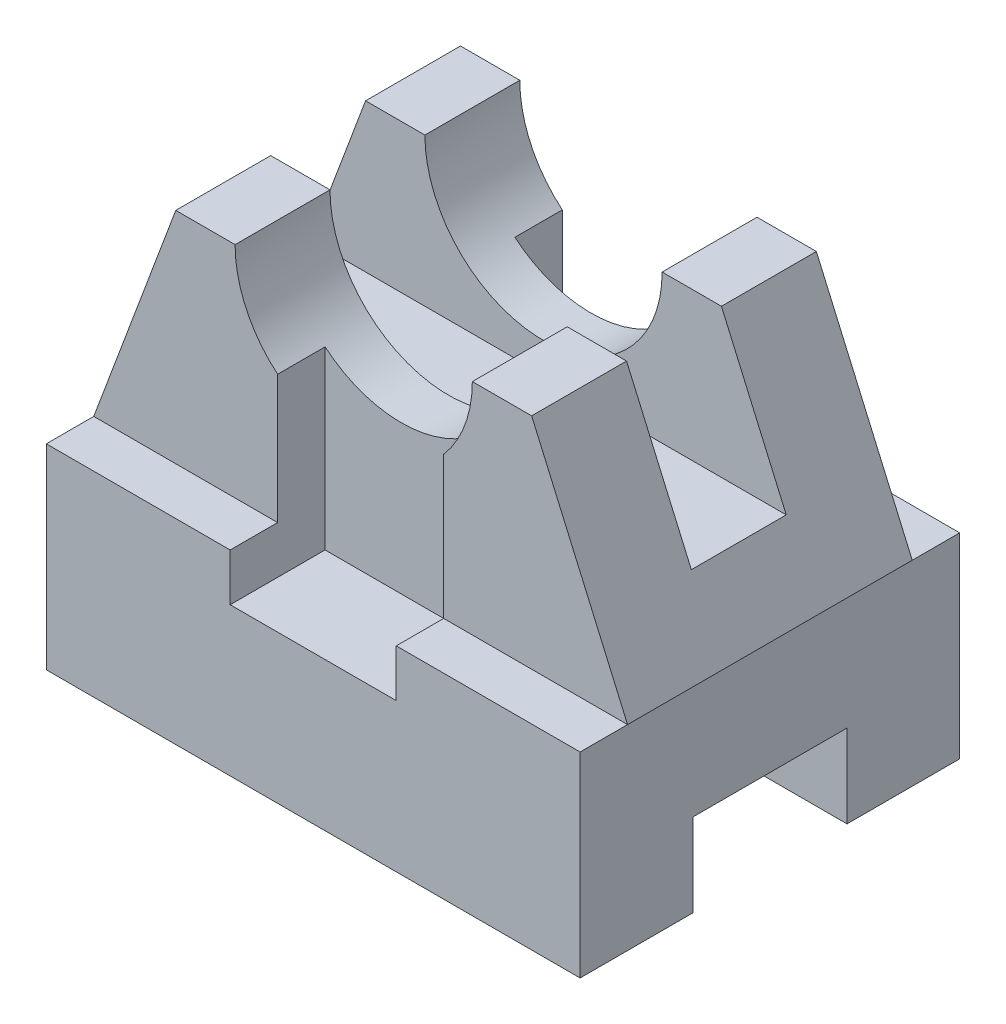
ISO-10303-21;
HEADER;
FILE_DESCRIPTION(('STEP AP214'),'2;1');
FILE_NAME('part.step','',(''),(''),'','','');
FILE_SCHEMA(('AUTOMOTIVE_DESIGN { 1 0 10303 214 1 1 1 1 }'));
ENDSEC;
DATA;
#1=APPLICATION_CONTEXT('core data for automotive mechanical design processes');
#2=APPLICATION_PROTOCOL_DEFINITION('international standard','automotive_design',2000,#1);
#3=PRODUCT_CONTEXT('',#1,'mechanical');
#4=PRODUCT('Part','Part','',(#3));
#5=PRODUCT_RELATED_PRODUCT_CATEGORY('part','',(#4));
#6=PRODUCT_DEFINITION_FORMATION('','',#4);
#7=PRODUCT_DEFINITION_CONTEXT('part definition',#1,'design');
#8=PRODUCT_DEFINITION('design','',#6,#7);
#9=PRODUCT_DEFINITION_SHAPE('','',#8);
#10=(LENGTH_UNIT() NAMED_UNIT(*) SI_UNIT(.MILLI.,.METRE.));
#11=(NAMED_UNIT(*) PLANE_ANGLE_UNIT() SI_UNIT($,.RADIAN.));
#12=(NAMED_UNIT(*) SI_UNIT($,.STERADIAN.) SOLID_ANGLE_UNIT());
#13=UNCERTAINTY_MEASURE_WITH_UNIT(LENGTH_MEASURE(1.E-05),#10,'distance_accuracy_value','');
#14=(GEOMETRIC_REPRESENTATION_CONTEXT(3) GLOBAL_UNCERTAINTY_ASSIGNED_CONTEXT((#13)) GLOBAL_UNIT_ASSIGNED_CONTEXT((#10,
#11,#12)) REPRESENTATION_CONTEXT('',''));
#15=CARTESIAN_POINT('',(0.,0.,0.));
#16=DIRECTION('',(0.,0.,1.));
#17=DIRECTION('',(1.,0.,0.));
#18=AXIS2_PLACEMENT_3D('',#15,#16,#17);
#19=CARTESIAN_POINT('',(0.,33.,32.));
#20=DIRECTION('',(0.,-1.,0.));
#21=DIRECTION('',(0.,0.,-1.));
#22=AXIS2_PLACEMENT_3D('',#19,#20,#21);
#23=PLANE('',#22);
#24=DIRECTION('',(-1.,0.,0.));
#25=VECTOR('',#24,1.);
#26=CARTESIAN_POINT('',(0.,33.,32.));
#27=LINE('',#26,#25);
#28=CARTESIAN_POINT('',(31.,33.,32.));
#29=VERTEX_POINT('',#28);
#30=CARTESIAN_POINT('',(0.,33.,32.));
#31=VERTEX_POINT('',#30);
#32=EDGE_CURVE('E433',#29,#31,#27,.T.);
#33=ORIENTED_EDGE('',*,*,#32,.F.);
#34=DIRECTION('',(0.,0.,-1.));
#35=VECTOR('',#34,1.);
#36=CARTESIAN_POINT('',(31.,33.,32.));
#37=LINE('',#36,#35);
#38=CARTESIAN_POINT('',(31.,33.,24.));
#39=VERTEX_POINT('',#38);
#40=EDGE_CURVE('E304',#29,#39,#37,.T.);
#41=ORIENTED_EDGE('',*,*,#40,.T.);
#42=DIRECTION('',(1.,0.,0.));
#43=VECTOR('',#42,1.);
#44=CARTESIAN_POINT('',(0.,33.,24.));
#45=LINE('',#44,#43);
#46=CARTESIAN_POINT('',(0.,33.,24.));
#47=VERTEX_POINT('',#46);
#48=EDGE_CURVE('E398',#47,#39,#45,.T.);
#49=ORIENTED_EDGE('',*,*,#48,.F.);
#50=DIRECTION('',(0.,0.,-1.));
#51=VECTOR('',#50,1.);
#52=CARTESIAN_POINT('',(0.,33.,32.));
#53=LINE('',#52,#51);
#54=EDGE_CURVE('E449',#31,#47,#53,.T.);
#55=ORIENTED_EDGE('',*,*,#54,.F.);
#56=EDGE_LOOP('',(#33,#41,#49,#55));
#57=FACE_BOUND('',#56,.T.);
#58=ADVANCED_FACE('F39',(#57),#23,.F.);
#59=DIRECTION('',(1.,0.,0.));
#60=VECTOR('',#59,1.);
#61=CARTESIAN_POINT('',(0.,33.,-24.));
#62=LINE('',#61,#60);
#63=CARTESIAN_POINT('',(0.,33.,-24.));
#64=VERTEX_POINT('',#63);
#65=CARTESIAN_POINT('',(31.,33.,-24.));
#66=VERTEX_POINT('',#65);
#67=EDGE_CURVE('E395',#64,#66,#62,.T.);
#68=ORIENTED_EDGE('',*,*,#67,.T.);
#69=DIRECTION('',(0.,0.,-1.));
#70=VECTOR('',#69,1.);
#71=CARTESIAN_POINT('',(31.,33.,32.));
#72=LINE('',#71,#70);
#73=CARTESIAN_POINT('',(31.,33.,-32.));
#74=VERTEX_POINT('',#73);
#75=EDGE_CURVE('E312',#66,#74,#72,.T.);
#76=ORIENTED_EDGE('',*,*,#75,.T.);
#77=DIRECTION('',(-1.,0.,0.));
#78=VECTOR('',#77,1.);
#79=CARTESIAN_POINT('',(0.,33.,-32.));
#80=LINE('',#79,#78);
#81=CARTESIAN_POINT('',(0.,33.,-32.));
#82=VERTEX_POINT('',#81);
#83=EDGE_CURVE('E448',#74,#82,#80,.T.);
#84=ORIENTED_EDGE('',*,*,#83,.T.);
#85=EDGE_CURVE('E440',#64,#82,#53,.T.);
#86=ORIENTED_EDGE('',*,*,#85,.F.);
#87=EDGE_LOOP('',(#68,#76,#84,#86));
#88=FACE_BOUND('',#87,.T.);
#89=ADVANCED_FACE('F541',(#88),#23,.F.);
#90=CARTESIAN_POINT('',(0.,33.,24.));
#91=DIRECTION('',(0.,0.,1.));
#92=DIRECTION('',(1.,0.,0.));
#93=AXIS2_PLACEMENT_3D('',#90,#91,#92);
#94=PLANE('',#93);
#95=DIRECTION('',(0.,-1.,0.));
#96=VECTOR('',#95,1.);
#97=CARTESIAN_POINT('',(31.,33.,24.));
#98=LINE('',#97,#96);
#99=CARTESIAN_POINT('',(31.,54.6572138549099,24.));
#100=VERTEX_POINT('',#99);
#101=EDGE_CURVE('E301',#100,#39,#98,.T.);
#102=ORIENTED_EDGE('',*,*,#101,.F.);
#103=CARTESIAN_POINT('',(43.8296108010349,70.,24.));
#104=DIRECTION('',(0.,0.,1.));
#105=DIRECTION('',(1.,0.,0.));
#106=AXIS2_PLACEMENT_3D('',#103,#104,#105);
#107=CIRCLE('',#106,20.);
#108=CARTESIAN_POINT('',(23.8296108010349,70.,24.));
#109=VERTEX_POINT('',#108);
#110=EDGE_CURVE('E331',#109,#100,#107,.T.);
#111=ORIENTED_EDGE('',*,*,#110,.F.);
#112=DIRECTION('',(1.,0.,0.));
#113=VECTOR('',#112,1.);
#114=CARTESIAN_POINT('',(0.,70.,24.));
#115=LINE('',#114,#113);
#116=CARTESIAN_POINT('',(13.8296108010349,70.,24.));
#117=VERTEX_POINT('',#116);
#118=EDGE_CURVE('E369',#117,#109,#115,.T.);
#119=ORIENTED_EDGE('',*,*,#118,.F.);
#120=DIRECTION('',(0.350115816415792,0.936706418839704,0.));
#121=VECTOR('',#120,1.);
#122=CARTESIAN_POINT('',(-10.8225391749412,4.04517580184839,24.));
#123=LINE('',#122,#121);
#124=EDGE_CURVE('E340',#47,#117,#123,.T.);
#125=ORIENTED_EDGE('',*,*,#124,.F.);
#126=ORIENTED_EDGE('',*,*,#48,.T.);
#127=EDGE_LOOP('',(#102,#111,#119,#125,#126));
#128=FACE_BOUND('',#127,.T.);
#129=ADVANCED_FACE('F603',(#128),#94,.T.);
#130=CARTESIAN_POINT('',(0.,33.,-24.));
#131=DIRECTION('',(0.,0.,-1.));
#132=DIRECTION('',(-1.,0.,0.));
#133=AXIS2_PLACEMENT_3D('',#130,#131,#132);
#134=PLANE('',#133);
#135=DIRECTION('',(0.,1.,0.));
#136=VECTOR('',#135,1.);
#137=CARTESIAN_POINT('',(31.,33.,-24.));
#138=LINE('',#137,#136);
#139=CARTESIAN_POINT('',(31.,54.6572138549099,-24.));
#140=VERTEX_POINT('',#139);
#141=EDGE_CURVE('E311',#66,#140,#138,.T.);
#142=ORIENTED_EDGE('',*,*,#141,.F.);
#143=ORIENTED_EDGE('',*,*,#67,.F.);
#144=DIRECTION('',(-0.350115816415792,-0.936706418839704,0.));
#145=VECTOR('',#144,1.);
#146=CARTESIAN_POINT('',(0.,33.,-24.));
#147=LINE('',#146,#145);
#148=CARTESIAN_POINT('',(13.8296108010349,70.,-24.));
#149=VERTEX_POINT('',#148);
#150=EDGE_CURVE('E464',#149,#64,#147,.T.);
#151=ORIENTED_EDGE('',*,*,#150,.F.);
#152=DIRECTION('',(1.,0.,0.));
#153=VECTOR('',#152,1.);
#154=CARTESIAN_POINT('',(0.,70.,-24.));
#155=LINE('',#154,#153);
#156=CARTESIAN_POINT('',(23.8296108010349,70.,-24.));
#157=VERTEX_POINT('',#156);
#158=EDGE_CURVE('E389',#149,#157,#155,.T.);
#159=ORIENTED_EDGE('',*,*,#158,.T.);
#160=CARTESIAN_POINT('',(43.8296108010349,70.,-24.));
#161=DIRECTION('',(0.,0.,-1.));
#162=DIRECTION('',(-1.,0.,0.));
#163=AXIS2_PLACEMENT_3D('',#160,#161,#162);
#164=CIRCLE('',#163,20.);
#165=EDGE_CURVE('E318',#140,#157,#164,.T.);
#166=ORIENTED_EDGE('',*,*,#165,.F.);
#167=EDGE_LOOP('',(#142,#143,#151,#159,#166));
#168=FACE_BOUND('',#167,.T.);
#169=ADVANCED_FACE('F550',(#168),#134,.T.);
#170=CARTESIAN_POINT('',(0.,70.,24.));
#171=DIRECTION('',(0.,1.,0.));
#172=DIRECTION('',(0.,0.,1.));
#173=AXIS2_PLACEMENT_3D('',#170,#171,#172);
#174=PLANE('',#173);
#175=DIRECTION('',(0.,0.,-1.));
#176=VECTOR('',#175,1.);
#177=CARTESIAN_POINT('',(63.8296108010349,70.,32.));
#178=LINE('',#177,#176);
#179=CARTESIAN_POINT('',(63.8296108010349,70.,24.));
#180=VERTEX_POINT('',#179);
#181=CARTESIAN_POINT('',(63.8296108010349,70.,8.));
#182=VERTEX_POINT('',#181);
#183=EDGE_CURVE('E324',#180,#182,#178,.T.);
#184=ORIENTED_EDGE('',*,*,#183,.F.);
#185=CARTESIAN_POINT('',(73.8296108010349,70.,24.));
#186=VERTEX_POINT('',#185);
#187=EDGE_CURVE('E373',#180,#186,#115,.T.);
#188=ORIENTED_EDGE('',*,*,#187,.T.);
#189=DIRECTION('',(0.,0.,1.));
#190=VECTOR('',#189,1.);
#191=CARTESIAN_POINT('',(73.8296108010349,70.,-32.));
#192=LINE('',#191,#190);
#193=CARTESIAN_POINT('',(73.8296108010349,70.,8.));
#194=VERTEX_POINT('',#193);
#195=EDGE_CURVE('E343',#194,#186,#192,.T.);
#196=ORIENTED_EDGE('',*,*,#195,.F.);
#197=DIRECTION('',(1.,0.,0.));
#198=VECTOR('',#197,1.);
#199=CARTESIAN_POINT('',(0.,70.,8.));
#200=LINE('',#199,#198);
#201=EDGE_CURVE('E380',#182,#194,#200,.T.);
#202=ORIENTED_EDGE('',*,*,#201,.F.);
#203=EDGE_LOOP('',(#184,#188,#196,#202));
#204=FACE_BOUND('',#203,.T.);
#205=ADVANCED_FACE('F576',(#204),#174,.T.);
#206=CARTESIAN_POINT('',(0.,70.,-8.));
#207=DIRECTION('',(0.,1.,0.));
#208=DIRECTION('',(0.,0.,1.));
#209=AXIS2_PLACEMENT_3D('',#206,#207,#208);
#210=PLANE('',#209);
#211=CARTESIAN_POINT('',(63.8296108010349,70.,-8.));
#212=VERTEX_POINT('',#211);
#213=CARTESIAN_POINT('',(63.8296108010349,70.,-24.));
#214=VERTEX_POINT('',#213);
#215=EDGE_CURVE('E323',#212,#214,#178,.T.);
#216=ORIENTED_EDGE('',*,*,#215,.F.);
#217=DIRECTION('',(1.,0.,0.));
#218=VECTOR('',#217,1.);
#219=CARTESIAN_POINT('',(0.,70.,-8.));
#220=LINE('',#219,#218);
#221=CARTESIAN_POINT('',(73.8296108010349,70.,-8.));
#222=VERTEX_POINT('',#221);
#223=EDGE_CURVE('E390',#212,#222,#220,.T.);
#224=ORIENTED_EDGE('',*,*,#223,.T.);
#225=CARTESIAN_POINT('',(73.8296108010349,70.,-24.));
#226=VERTEX_POINT('',#225);
#227=EDGE_CURVE('E350',#226,#222,#192,.T.);
#228=ORIENTED_EDGE('',*,*,#227,.F.);
#229=EDGE_CURVE('E393',#214,#226,#155,.T.);
#230=ORIENTED_EDGE('',*,*,#229,.F.);
#231=EDGE_LOOP('',(#216,#224,#228,#230));
#232=FACE_BOUND('',#231,.T.);
#233=ADVANCED_FACE('F561',(#232),#210,.T.);
#234=CARTESIAN_POINT('',(59.,33.,24.));
#235=VERTEX_POINT('',#234);
#236=CARTESIAN_POINT('',(90.,33.,24.));
#237=VERTEX_POINT('',#236);
#238=EDGE_CURVE('E366',#235,#237,#45,.T.);
#239=ORIENTED_EDGE('',*,*,#238,.F.);
#240=DIRECTION('',(0.,0.,1.));
#241=VECTOR('',#240,1.);
#242=CARTESIAN_POINT('',(59.,33.,32.));
#243=LINE('',#242,#241);
#244=CARTESIAN_POINT('',(59.,33.,32.));
#245=VERTEX_POINT('',#244);
#246=EDGE_CURVE('E297',#235,#245,#243,.T.);
#247=ORIENTED_EDGE('',*,*,#246,.T.);
#248=CARTESIAN_POINT('',(90.,33.,32.));
#249=VERTEX_POINT('',#248);
#250=EDGE_CURVE('E432',#249,#245,#27,.T.);
#251=ORIENTED_EDGE('',*,*,#250,.F.);
#252=DIRECTION('',(0.,0.,-1.));
#253=VECTOR('',#252,1.);
#254=CARTESIAN_POINT('',(90.,33.,32.));
#255=LINE('',#254,#253);
#256=EDGE_CURVE('E451',#249,#237,#255,.T.);
#257=ORIENTED_EDGE('',*,*,#256,.T.);
#258=EDGE_LOOP('',(#239,#247,#251,#257));
#259=FACE_BOUND('',#258,.T.);
#260=ADVANCED_FACE('F508',(#259),#23,.F.);
#261=CARTESIAN_POINT('',(0.,0.,32.));
#262=DIRECTION('',(0.,1.,0.));
#263=DIRECTION('',(0.,0.,1.));
#264=AXIS2_PLACEMENT_3D('',#261,#262,#263);
#265=PLANE('',#264);
#266=DIRECTION('',(0.,0.,-1.));
#267=VECTOR('',#266,1.);
#268=CARTESIAN_POINT('',(0.,0.,32.));
#269=LINE('',#268,#267);
#270=CARTESIAN_POINT('',(0.,0.,32.));
#271=VERTEX_POINT('',#270);
#272=CARTESIAN_POINT('',(0.,0.,13.));
#273=VERTEX_POINT('',#272);
#274=EDGE_CURVE('E463',#271,#273,#269,.T.);
#275=ORIENTED_EDGE('',*,*,#274,.T.);
#276=DIRECTION('',(1.,0.,0.));
#277=VECTOR('',#276,1.);
#278=CARTESIAN_POINT('',(0.,0.,13.));
#279=LINE('',#278,#277);
#280=CARTESIAN_POINT('',(90.,0.,13.));
#281=VERTEX_POINT('',#280);
#282=EDGE_CURVE('E409',#273,#281,#279,.T.);
#283=ORIENTED_EDGE('',*,*,#282,.T.);
#284=DIRECTION('',(0.,0.,-1.));
#285=VECTOR('',#284,1.);
#286=CARTESIAN_POINT('',(90.,0.,32.));
#287=LINE('',#286,#285);
#288=CARTESIAN_POINT('',(90.,0.,32.));
#289=VERTEX_POINT('',#288);
#290=EDGE_CURVE('E460',#289,#281,#287,.T.);
#291=ORIENTED_EDGE('',*,*,#290,.F.);
#292=DIRECTION('',(1.,0.,0.));
#293=VECTOR('',#292,1.);
#294=CARTESIAN_POINT('',(0.,0.,32.));
#295=LINE('',#294,#293);
#296=EDGE_CURVE('E428',#271,#289,#295,.T.);
#297=ORIENTED_EDGE('',*,*,#296,.F.);
#298=EDGE_LOOP('',(#275,#283,#291,#297));
#299=FACE_BOUND('',#298,.T.);
#300=ADVANCED_FACE('F513',(#299),#265,.F.);
#301=CARTESIAN_POINT('',(0.,0.,32.));
#302=DIRECTION('',(1.,0.,0.));
#303=DIRECTION('',(0.,0.,-1.));
#304=AXIS2_PLACEMENT_3D('',#301,#302,#303);
#305=PLANE('',#304);
#306=ORIENTED_EDGE('',*,*,#54,.T.);
#307=DIRECTION('',(0.,0.,1.));
#308=VECTOR('',#307,1.);
#309=CARTESIAN_POINT('',(0.,33.,-32.));
#310=LINE('',#309,#308);
#311=EDGE_CURVE('E353',#64,#47,#310,.T.);
#312=ORIENTED_EDGE('',*,*,#311,.F.);
#313=ORIENTED_EDGE('',*,*,#85,.T.);
#314=DIRECTION('',(0.,-1.,0.));
#315=VECTOR('',#314,1.);
#316=CARTESIAN_POINT('',(0.,0.,-32.));
#317=LINE('',#316,#315);
#318=CARTESIAN_POINT('',(0.,0.,-32.));
#319=VERTEX_POINT('',#318);
#320=EDGE_CURVE('E416',#82,#319,#317,.T.);
#321=ORIENTED_EDGE('',*,*,#320,.T.);
#322=CARTESIAN_POINT('',(0.,0.,-13.));
#323=VERTEX_POINT('',#322);
#324=EDGE_CURVE('E458',#323,#319,#269,.T.);
#325=ORIENTED_EDGE('',*,*,#324,.F.);
#326=DIRECTION('',(0.,1.,0.));
#327=VECTOR('',#326,1.);
#328=CARTESIAN_POINT('',(0.,0.,-13.));
#329=LINE('',#328,#327);
#330=CARTESIAN_POINT('',(0.,14.,-13.));
#331=VERTEX_POINT('',#330);
#332=EDGE_CURVE('E405',#323,#331,#329,.T.);
#333=ORIENTED_EDGE('',*,*,#332,.T.);
#334=DIRECTION('',(0.,0.,1.));
#335=VECTOR('',#334,1.);
#336=CARTESIAN_POINT('',(0.,14.,13.));
#337=LINE('',#336,#335);
#338=CARTESIAN_POINT('',(0.,14.,13.));
#339=VERTEX_POINT('',#338);
#340=EDGE_CURVE('E408',#331,#339,#337,.T.);
#341=ORIENTED_EDGE('',*,*,#340,.T.);
#342=DIRECTION('',(0.,-1.,0.));
#343=VECTOR('',#342,1.);
#344=CARTESIAN_POINT('',(0.,0.,13.));
#345=LINE('',#344,#343);
#346=EDGE_CURVE('E397',#339,#273,#345,.T.);
#347=ORIENTED_EDGE('',*,*,#346,.T.);
#348=ORIENTED_EDGE('',*,*,#274,.F.);
#349=DIRECTION('',(0.,-1.,0.));
#350=VECTOR('',#349,1.);
#351=CARTESIAN_POINT('',(0.,0.,32.));
#352=LINE('',#351,#350);
#353=EDGE_CURVE('E422',#31,#271,#352,.T.);
#354=ORIENTED_EDGE('',*,*,#353,.F.);
#355=EDGE_LOOP('',(#306,#312,#313,#321,#325,#333,#341,#347,#348,#354));
#356=FACE_BOUND('',#355,.T.);
#357=ADVANCED_FACE('F41',(#356),#305,.F.);
#358=CARTESIAN_POINT('',(90.,0.,-13.));
#359=VERTEX_POINT('',#358);
#360=CARTESIAN_POINT('',(90.,0.,-32.));
#361=VERTEX_POINT('',#360);
#362=EDGE_CURVE('E457',#359,#361,#287,.T.);
#363=ORIENTED_EDGE('',*,*,#362,.F.);
#364=DIRECTION('',(1.,0.,0.));
#365=VECTOR('',#364,1.);
#366=CARTESIAN_POINT('',(0.,0.,-13.));
#367=LINE('',#366,#365);
#368=EDGE_CURVE('E423',#323,#359,#367,.T.);
#369=ORIENTED_EDGE('',*,*,#368,.F.);
#370=ORIENTED_EDGE('',*,*,#324,.T.);
#371=DIRECTION('',(1.,0.,0.));
#372=VECTOR('',#371,1.);
#373=CARTESIAN_POINT('',(0.,0.,-32.));
#374=LINE('',#373,#372);
#375=EDGE_CURVE('E439',#319,#361,#374,.T.);
#376=ORIENTED_EDGE('',*,*,#375,.T.);
#377=EDGE_LOOP('',(#363,#369,#370,#376));
#378=FACE_BOUND('',#377,.T.);
#379=ADVANCED_FACE('F533',(#378),#265,.F.);
#380=CARTESIAN_POINT('',(90.,0.,32.));
#381=DIRECTION('',(-1.,0.,0.));
#382=DIRECTION('',(0.,0.,1.));
#383=AXIS2_PLACEMENT_3D('',#380,#381,#382);
#384=PLANE('',#383);
#385=CARTESIAN_POINT('',(90.,33.,-24.));
#386=VERTEX_POINT('',#385);
#387=CARTESIAN_POINT('',(90.,33.,-32.));
#388=VERTEX_POINT('',#387);
#389=EDGE_CURVE('E455',#386,#388,#255,.T.);
#390=ORIENTED_EDGE('',*,*,#389,.F.);
#391=DIRECTION('',(0.,0.,1.));
#392=VECTOR('',#391,1.);
#393=CARTESIAN_POINT('',(90.,33.,-32.));
#394=LINE('',#393,#392);
#395=EDGE_CURVE('E341',#386,#237,#394,.T.);
#396=ORIENTED_EDGE('',*,*,#395,.T.);
#397=ORIENTED_EDGE('',*,*,#256,.F.);
#398=DIRECTION('',(0.,1.,0.));
#399=VECTOR('',#398,1.);
#400=CARTESIAN_POINT('',(90.,0.,32.));
#401=LINE('',#400,#399);
#402=EDGE_CURVE('E431',#289,#249,#401,.T.);
#403=ORIENTED_EDGE('',*,*,#402,.F.);
#404=ORIENTED_EDGE('',*,*,#290,.T.);
#405=DIRECTION('',(0.,-1.,0.));
#406=VECTOR('',#405,1.);
#407=CARTESIAN_POINT('',(90.,0.,13.));
#408=LINE('',#407,#406);
#409=CARTESIAN_POINT('',(90.,14.,13.));
#410=VERTEX_POINT('',#409);
#411=EDGE_CURVE('E375',#410,#281,#408,.T.);
#412=ORIENTED_EDGE('',*,*,#411,.F.);
#413=DIRECTION('',(0.,0.,1.));
#414=VECTOR('',#413,1.);
#415=CARTESIAN_POINT('',(90.,14.,13.));
#416=LINE('',#415,#414);
#417=CARTESIAN_POINT('',(90.,14.,-13.));
#418=VERTEX_POINT('',#417);
#419=EDGE_CURVE('E401',#418,#410,#416,.T.);
#420=ORIENTED_EDGE('',*,*,#419,.F.);
#421=DIRECTION('',(0.,1.,0.));
#422=VECTOR('',#421,1.);
#423=CARTESIAN_POINT('',(90.,0.,-13.));
#424=LINE('',#423,#422);
#425=EDGE_CURVE('E413',#359,#418,#424,.T.);
#426=ORIENTED_EDGE('',*,*,#425,.F.);
#427=ORIENTED_EDGE('',*,*,#362,.T.);
#428=DIRECTION('',(0.,1.,0.));
#429=VECTOR('',#428,1.);
#430=CARTESIAN_POINT('',(90.,0.,-32.));
#431=LINE('',#430,#429);
#432=EDGE_CURVE('E444',#361,#388,#431,.T.);
#433=ORIENTED_EDGE('',*,*,#432,.T.);
#434=EDGE_LOOP('',(#390,#396,#397,#403,#404,#412,#420,#426,#427,#433));
#435=FACE_BOUND('',#434,.T.);
#436=ADVANCED_FACE('F503',(#435),#384,.F.);
#437=CARTESIAN_POINT('',(59.,33.,-32.));
#438=VERTEX_POINT('',#437);
#439=EDGE_CURVE('E427',#388,#438,#80,.T.);
#440=ORIENTED_EDGE('',*,*,#439,.T.);
#441=DIRECTION('',(0.,0.,1.));
#442=VECTOR('',#441,1.);
#443=CARTESIAN_POINT('',(59.,33.,32.));
#444=LINE('',#443,#442);
#445=CARTESIAN_POINT('',(59.,33.,-24.));
#446=VERTEX_POINT('',#445);
#447=EDGE_CURVE('E309',#438,#446,#444,.T.);
#448=ORIENTED_EDGE('',*,*,#447,.T.);
#449=EDGE_CURVE('E392',#446,#386,#62,.T.);
#450=ORIENTED_EDGE('',*,*,#449,.T.);
#451=ORIENTED_EDGE('',*,*,#389,.T.);
#452=EDGE_LOOP('',(#440,#448,#450,#451));
#453=FACE_BOUND('',#452,.T.);
#454=ADVANCED_FACE('F492',(#453),#23,.F.);
#455=CARTESIAN_POINT('',(0.,0.,32.));
#456=DIRECTION('',(0.,0.,-1.));
#457=DIRECTION('',(-1.,0.,0.));
#458=AXIS2_PLACEMENT_3D('',#455,#456,#457);
#459=PLANE('',#458);
#460=DIRECTION('',(1.,0.,0.));
#461=VECTOR('',#460,1.);
#462=CARTESIAN_POINT('',(31.,25.,32.));
#463=LINE('',#462,#461);
#464=CARTESIAN_POINT('',(31.,25.,32.));
#465=VERTEX_POINT('',#464);
#466=CARTESIAN_POINT('',(59.,25.,32.));
#467=VERTEX_POINT('',#466);
#468=EDGE_CURVE('E267',#465,#467,#463,.T.);
#469=ORIENTED_EDGE('',*,*,#468,.F.);
#470=DIRECTION('',(0.,1.,0.));
#471=VECTOR('',#470,1.);
#472=CARTESIAN_POINT('',(31.,25.,32.));
#473=LINE('',#472,#471);
#474=EDGE_CURVE('E278',#465,#29,#473,.T.);
#475=ORIENTED_EDGE('',*,*,#474,.T.);
#476=ORIENTED_EDGE('',*,*,#32,.T.);
#477=ORIENTED_EDGE('',*,*,#353,.T.);
#478=ORIENTED_EDGE('',*,*,#296,.T.);
#479=ORIENTED_EDGE('',*,*,#402,.T.);
#480=ORIENTED_EDGE('',*,*,#250,.T.);
#481=DIRECTION('',(0.,1.,0.));
#482=VECTOR('',#481,1.);
#483=CARTESIAN_POINT('',(59.,25.,32.));
#484=LINE('',#483,#482);
#485=EDGE_CURVE('E284',#467,#245,#484,.T.);
#486=ORIENTED_EDGE('',*,*,#485,.F.);
#487=EDGE_LOOP('',(#469,#475,#476,#477,#478,#479,#480,#486));
#488=FACE_BOUND('',#487,.T.);
#489=ADVANCED_FACE('F509',(#488),#459,.F.);
#490=CARTESIAN_POINT('',(0.,0.,-32.));
#491=DIRECTION('',(0.,0.,-1.));
#492=DIRECTION('',(-1.,0.,0.));
#493=AXIS2_PLACEMENT_3D('',#490,#491,#492);
#494=PLANE('',#493);
#495=DIRECTION('',(0.,1.,0.));
#496=VECTOR('',#495,1.);
#497=CARTESIAN_POINT('',(31.,25.,-32.));
#498=LINE('',#497,#496);
#499=CARTESIAN_POINT('',(31.,25.,-32.));
#500=VERTEX_POINT('',#499);
#501=EDGE_CURVE('E273',#500,#74,#498,.T.);
#502=ORIENTED_EDGE('',*,*,#501,.F.);
#503=DIRECTION('',(-1.,0.,0.));
#504=VECTOR('',#503,1.);
#505=CARTESIAN_POINT('',(31.,25.,-32.));
#506=LINE('',#505,#504);
#507=CARTESIAN_POINT('',(59.,25.,-32.));
#508=VERTEX_POINT('',#507);
#509=EDGE_CURVE('E252',#508,#500,#506,.T.);
#510=ORIENTED_EDGE('',*,*,#509,.F.);
#511=DIRECTION('',(0.,1.,0.));
#512=VECTOR('',#511,1.);
#513=CARTESIAN_POINT('',(59.,25.,-32.));
#514=LINE('',#513,#512);
#515=EDGE_CURVE('E277',#508,#438,#514,.T.);
#516=ORIENTED_EDGE('',*,*,#515,.T.);
#517=ORIENTED_EDGE('',*,*,#439,.F.);
#518=ORIENTED_EDGE('',*,*,#432,.F.);
#519=ORIENTED_EDGE('',*,*,#375,.F.);
#520=ORIENTED_EDGE('',*,*,#320,.F.);
#521=ORIENTED_EDGE('',*,*,#83,.F.);
#522=EDGE_LOOP('',(#502,#510,#516,#517,#518,#519,#520,#521));
#523=FACE_BOUND('',#522,.T.);
#524=ADVANCED_FACE('F540',(#523),#494,.T.);
#525=CARTESIAN_POINT('',(0.,0.,13.));
#526=DIRECTION('',(0.,0.,1.));
#527=DIRECTION('',(0.,-1.,0.));
#528=AXIS2_PLACEMENT_3D('',#525,#526,#527);
#529=PLANE('',#528);
#530=ORIENTED_EDGE('',*,*,#411,.T.);
#531=ORIENTED_EDGE('',*,*,#282,.F.);
#532=ORIENTED_EDGE('',*,*,#346,.F.);
#533=DIRECTION('',(1.,0.,0.));
#534=VECTOR('',#533,1.);
#535=CARTESIAN_POINT('',(0.,14.,13.));
#536=LINE('',#535,#534);
#537=EDGE_CURVE('E418',#339,#410,#536,.T.);
#538=ORIENTED_EDGE('',*,*,#537,.T.);
#539=EDGE_LOOP('',(#530,#531,#532,#538));
#540=FACE_BOUND('',#539,.T.);
#541=ADVANCED_FACE('F519',(#540),#529,.F.);
#542=CARTESIAN_POINT('',(0.,14.,13.));
#543=DIRECTION('',(0.,1.,0.));
#544=DIRECTION('',(0.,0.,1.));
#545=AXIS2_PLACEMENT_3D('',#542,#543,#544);
#546=PLANE('',#545);
#547=ORIENTED_EDGE('',*,*,#419,.T.);
#548=ORIENTED_EDGE('',*,*,#537,.F.);
#549=ORIENTED_EDGE('',*,*,#340,.F.);
#550=DIRECTION('',(1.,0.,0.));
#551=VECTOR('',#550,1.);
#552=CARTESIAN_POINT('',(0.,14.,-13.));
#553=LINE('',#552,#551);
#554=EDGE_CURVE('E420',#331,#418,#553,.T.);
#555=ORIENTED_EDGE('',*,*,#554,.T.);
#556=EDGE_LOOP('',(#547,#548,#549,#555));
#557=FACE_BOUND('',#556,.T.);
#558=ADVANCED_FACE('F524',(#557),#546,.F.);
#559=CARTESIAN_POINT('',(0.,0.,-13.));
#560=DIRECTION('',(0.,0.,-1.));
#561=DIRECTION('',(0.,1.,0.));
#562=AXIS2_PLACEMENT_3D('',#559,#560,#561);
#563=PLANE('',#562);
#564=ORIENTED_EDGE('',*,*,#425,.T.);
#565=ORIENTED_EDGE('',*,*,#554,.F.);
#566=ORIENTED_EDGE('',*,*,#332,.F.);
#567=ORIENTED_EDGE('',*,*,#368,.T.);
#568=EDGE_LOOP('',(#564,#565,#566,#567));
#569=FACE_BOUND('',#568,.T.);
#570=ADVANCED_FACE('F810',(#569),#563,.F.);
#571=DIRECTION('',(0.,1.,0.));
#572=VECTOR('',#571,1.);
#573=CARTESIAN_POINT('',(59.,33.,24.));
#574=LINE('',#573,#572);
#575=CARTESIAN_POINT('',(59.,56.9669922292694,24.));
#576=VERTEX_POINT('',#575);
#577=EDGE_CURVE('E65',#235,#576,#574,.T.);
#578=ORIENTED_EDGE('',*,*,#577,.F.);
#579=ORIENTED_EDGE('',*,*,#238,.T.);
#580=DIRECTION('',(0.400463129476874,-0.916312873384189,0.));
#581=VECTOR('',#580,1.);
#582=CARTESIAN_POINT('',(87.6759695618905,38.3176905733077,24.));
#583=LINE('',#582,#581);
#584=EDGE_CURVE('E336',#186,#237,#583,.T.);
#585=ORIENTED_EDGE('',*,*,#584,.F.);
#586=ORIENTED_EDGE('',*,*,#187,.F.);
#587=EDGE_CURVE('E334',#576,#180,#107,.T.);
#588=ORIENTED_EDGE('',*,*,#587,.F.);
#589=EDGE_LOOP('',(#578,#579,#585,#586,#588));
#590=FACE_BOUND('',#589,.T.);
#591=ADVANCED_FACE('F583',(#590),#94,.T.);
#592=DIRECTION('',(0.,0.,-1.));
#593=VECTOR('',#592,1.);
#594=CARTESIAN_POINT('',(23.8296108010349,70.,32.));
#595=LINE('',#594,#593);
#596=CARTESIAN_POINT('',(23.8296108010349,70.,8.));
#597=VERTEX_POINT('',#596);
#598=EDGE_CURVE('E326',#109,#597,#595,.T.);
#599=ORIENTED_EDGE('',*,*,#598,.T.);
#600=CARTESIAN_POINT('',(13.8296108010349,70.,8.));
#601=VERTEX_POINT('',#600);
#602=EDGE_CURVE('E372',#601,#597,#200,.T.);
#603=ORIENTED_EDGE('',*,*,#602,.F.);
#604=DIRECTION('',(0.,0.,1.));
#605=VECTOR('',#604,1.);
#606=CARTESIAN_POINT('',(13.8296108010349,70.,-32.));
#607=LINE('',#606,#605);
#608=EDGE_CURVE('E355',#601,#117,#607,.T.);
#609=ORIENTED_EDGE('',*,*,#608,.T.);
#610=ORIENTED_EDGE('',*,*,#118,.T.);
#611=EDGE_LOOP('',(#599,#603,#609,#610));
#612=FACE_BOUND('',#611,.T.);
#613=ADVANCED_FACE('F609',(#612),#174,.T.);
#614=CARTESIAN_POINT('',(0.,70.,8.));
#615=DIRECTION('',(0.,0.,-1.));
#616=DIRECTION('',(0.,1.,0.));
#617=AXIS2_PLACEMENT_3D('',#614,#615,#616);
#618=PLANE('',#617);
#619=CARTESIAN_POINT('',(43.8296108010349,70.,8.));
#620=DIRECTION('',(0.,0.,-1.));
#621=DIRECTION('',(0.,1.,0.));
#622=AXIS2_PLACEMENT_3D('',#619,#620,#621);
#623=CIRCLE('',#622,20.);
#624=EDGE_CURVE('E332',#182,#597,#623,.T.);
#625=ORIENTED_EDGE('',*,*,#624,.F.);
#626=ORIENTED_EDGE('',*,*,#201,.T.);
#627=DIRECTION('',(-0.400463129476874,0.916312873384189,0.));
#628=VECTOR('',#627,1.);
#629=CARTESIAN_POINT('',(61.9895031020139,97.0917403083789,8.00000000000001));
#630=LINE('',#629,#628);
#631=CARTESIAN_POINT('',(84.7555494489843,45.,8.));
#632=VERTEX_POINT('',#631);
#633=EDGE_CURVE('E364',#632,#194,#630,.T.);
#634=ORIENTED_EDGE('',*,*,#633,.F.);
#635=DIRECTION('',(1.,0.,0.));
#636=VECTOR('',#635,1.);
#637=CARTESIAN_POINT('',(0.,45.,8.));
#638=LINE('',#637,#636);
#639=CARTESIAN_POINT('',(4.48527917871403,45.,8.));
#640=VERTEX_POINT('',#639);
#641=EDGE_CURVE('E378',#640,#632,#638,.T.);
#642=ORIENTED_EDGE('',*,*,#641,.F.);
#643=DIRECTION('',(-0.350115816415792,-0.936706418839704,0.));
#644=VECTOR('',#643,1.);
#645=CARTESIAN_POINT('',(12.1343621052371,65.4644998585336,8.));
#646=LINE('',#645,#644);
#647=EDGE_CURVE('E357',#601,#640,#646,.T.);
#648=ORIENTED_EDGE('',*,*,#647,.F.);
#649=ORIENTED_EDGE('',*,*,#602,.T.);
#650=EDGE_LOOP('',(#625,#626,#634,#642,#648,#649));
#651=FACE_BOUND('',#650,.T.);
#652=ADVANCED_FACE('F571',(#651),#618,.T.);
#653=CARTESIAN_POINT('',(0.,45.,8.));
#654=DIRECTION('',(0.,1.,0.));
#655=DIRECTION('',(0.,0.,1.));
#656=AXIS2_PLACEMENT_3D('',#653,#654,#655);
#657=PLANE('',#656);
#658=DIRECTION('',(0.,0.,1.));
#659=VECTOR('',#658,1.);
#660=CARTESIAN_POINT('',(84.7555494489843,45.,8.));
#661=LINE('',#660,#659);
#662=CARTESIAN_POINT('',(84.7555494489843,45.,-8.));
#663=VERTEX_POINT('',#662);
#664=EDGE_CURVE('E361',#663,#632,#661,.T.);
#665=ORIENTED_EDGE('',*,*,#664,.F.);
#666=DIRECTION('',(1.,0.,0.));
#667=VECTOR('',#666,1.);
#668=CARTESIAN_POINT('',(0.,45.,-8.));
#669=LINE('',#668,#667);
#670=CARTESIAN_POINT('',(4.48527917871402,45.,-8.));
#671=VERTEX_POINT('',#670);
#672=EDGE_CURVE('E381',#671,#663,#669,.T.);
#673=ORIENTED_EDGE('',*,*,#672,.F.);
#674=DIRECTION('',(0.,0.,-1.));
#675=VECTOR('',#674,1.);
#676=CARTESIAN_POINT('',(4.48527917871403,45.,8.));
#677=LINE('',#676,#675);
#678=EDGE_CURVE('E360',#640,#671,#677,.T.);
#679=ORIENTED_EDGE('',*,*,#678,.F.);
#680=ORIENTED_EDGE('',*,*,#641,.T.);
#681=EDGE_LOOP('',(#665,#673,#679,#680));
#682=FACE_BOUND('',#681,.T.);
#683=ADVANCED_FACE('F570',(#682),#657,.T.);
#684=CARTESIAN_POINT('',(0.,70.,-8.));
#685=DIRECTION('',(0.,0.,1.));
#686=DIRECTION('',(0.,-1.,0.));
#687=AXIS2_PLACEMENT_3D('',#684,#685,#686);
#688=PLANE('',#687);
#689=CARTESIAN_POINT('',(43.8296108010349,70.,-8.));
#690=DIRECTION('',(0.,0.,1.));
#691=DIRECTION('',(0.,-1.,0.));
#692=AXIS2_PLACEMENT_3D('',#689,#690,#691);
#693=CIRCLE('',#692,20.);
#694=CARTESIAN_POINT('',(23.8296108010349,70.,-8.));
#695=VERTEX_POINT('',#694);
#696=EDGE_CURVE('E328',#695,#212,#693,.T.);
#697=ORIENTED_EDGE('',*,*,#696,.F.);
#698=CARTESIAN_POINT('',(13.8296108010349,70.,-8.));
#699=VERTEX_POINT('',#698);
#700=EDGE_CURVE('E383',#699,#695,#220,.T.);
#701=ORIENTED_EDGE('',*,*,#700,.F.);
#702=DIRECTION('',(0.350115816415792,0.936706418839704,0.));
#703=VECTOR('',#702,1.);
#704=CARTESIAN_POINT('',(12.1343621052371,65.4644998585336,-8.));
#705=LINE('',#704,#703);
#706=EDGE_CURVE('E347',#671,#699,#705,.T.);
#707=ORIENTED_EDGE('',*,*,#706,.F.);
#708=ORIENTED_EDGE('',*,*,#672,.T.);
#709=DIRECTION('',(0.400463129476874,-0.916312873384189,0.));
#710=VECTOR('',#709,1.);
#711=CARTESIAN_POINT('',(61.9895031020139,97.0917403083789,-8.));
#712=LINE('',#711,#710);
#713=EDGE_CURVE('E363',#222,#663,#712,.T.);
#714=ORIENTED_EDGE('',*,*,#713,.F.);
#715=ORIENTED_EDGE('',*,*,#223,.F.);
#716=EDGE_LOOP('',(#697,#701,#707,#708,#714,#715));
#717=FACE_BOUND('',#716,.T.);
#718=ADVANCED_FACE('F560',(#717),#688,.T.);
#719=EDGE_CURVE('E325',#695,#157,#595,.T.);
#720=ORIENTED_EDGE('',*,*,#719,.T.);
#721=ORIENTED_EDGE('',*,*,#158,.F.);
#722=EDGE_CURVE('E345',#149,#699,#607,.T.);
#723=ORIENTED_EDGE('',*,*,#722,.T.);
#724=ORIENTED_EDGE('',*,*,#700,.T.);
#725=EDGE_LOOP('',(#720,#721,#723,#724));
#726=FACE_BOUND('',#725,.T.);
#727=ADVANCED_FACE('F555',(#726),#210,.T.);
#728=DIRECTION('',(0.,-1.,0.));
#729=VECTOR('',#728,1.);
#730=CARTESIAN_POINT('',(59.,33.,-24.));
#731=LINE('',#730,#729);
#732=CARTESIAN_POINT('',(59.,56.9669922292695,-24.));
#733=VERTEX_POINT('',#732);
#734=EDGE_CURVE('E306',#733,#446,#731,.T.);
#735=ORIENTED_EDGE('',*,*,#734,.F.);
#736=EDGE_CURVE('E317',#214,#733,#164,.T.);
#737=ORIENTED_EDGE('',*,*,#736,.F.);
#738=ORIENTED_EDGE('',*,*,#229,.T.);
#739=DIRECTION('',(-0.400463129476874,0.916312873384189,0.));
#740=VECTOR('',#739,1.);
#741=CARTESIAN_POINT('',(75.5666353736629,66.0254568769841,-24.));
#742=LINE('',#741,#740);
#743=EDGE_CURVE('E468',#386,#226,#742,.T.);
#744=ORIENTED_EDGE('',*,*,#743,.F.);
#745=ORIENTED_EDGE('',*,*,#449,.F.);
#746=EDGE_LOOP('',(#735,#737,#738,#744,#745));
#747=FACE_BOUND('',#746,.T.);
#748=ADVANCED_FACE('F490',(#747),#134,.T.);
#749=CARTESIAN_POINT('',(-10.8225391749412,4.04517580184839,-32.));
#750=DIRECTION('',(0.936706418839704,-0.350115816415792,0.));
#751=DIRECTION('',(0.350115816415792,0.936706418839704,0.));
#752=AXIS2_PLACEMENT_3D('',#749,#750,#751);
#753=PLANE('',#752);
#754=ORIENTED_EDGE('',*,*,#647,.T.);
#755=ORIENTED_EDGE('',*,*,#678,.T.);
#756=ORIENTED_EDGE('',*,*,#706,.T.);
#757=ORIENTED_EDGE('',*,*,#722,.F.);
#758=ORIENTED_EDGE('',*,*,#150,.T.);
#759=ORIENTED_EDGE('',*,*,#311,.T.);
#760=ORIENTED_EDGE('',*,*,#124,.T.);
#761=ORIENTED_EDGE('',*,*,#608,.F.);
#762=EDGE_LOOP('',(#754,#755,#756,#757,#758,#759,#760,#761));
#763=FACE_BOUND('',#762,.T.);
#764=ADVANCED_FACE('F599',(#763),#753,.F.);
#765=CARTESIAN_POINT('',(87.6759695618905,38.3176905733077,-32.));
#766=DIRECTION('',(-0.916312873384189,-0.400463129476874,0.));
#767=DIRECTION('',(0.400463129476874,-0.916312873384189,0.));
#768=AXIS2_PLACEMENT_3D('',#765,#766,#767);
#769=PLANE('',#768);
#770=ORIENTED_EDGE('',*,*,#633,.T.);
#771=ORIENTED_EDGE('',*,*,#195,.T.);
#772=ORIENTED_EDGE('',*,*,#584,.T.);
#773=ORIENTED_EDGE('',*,*,#395,.F.);
#774=ORIENTED_EDGE('',*,*,#743,.T.);
#775=ORIENTED_EDGE('',*,*,#227,.T.);
#776=ORIENTED_EDGE('',*,*,#713,.T.);
#777=ORIENTED_EDGE('',*,*,#664,.T.);
#778=EDGE_LOOP('',(#770,#771,#772,#773,#774,#775,#776,#777));
#779=FACE_BOUND('',#778,.T.);
#780=ADVANCED_FACE('F494',(#779),#769,.F.);
#781=CARTESIAN_POINT('',(43.8296108010349,70.,32.));
#782=DIRECTION('',(0.,0.,-1.));
#783=DIRECTION('',(-1.,0.,0.));
#784=AXIS2_PLACEMENT_3D('',#781,#782,#783);
#785=CYLINDRICAL_SURFACE('',#784,20.);
#786=CARTESIAN_POINT('',(43.8296108010349,70.,-16.));
#787=DIRECTION('',(0.,0.,1.));
#788=DIRECTION('',(1.,0.,0.));
#789=AXIS2_PLACEMENT_3D('',#786,#787,#788);
#790=CIRCLE('',#789,20.);
#791=CARTESIAN_POINT('',(59.,56.9669922292694,-16.));
#792=VERTEX_POINT('',#791);
#793=CARTESIAN_POINT('',(31.,54.6572138549099,-16.));
#794=VERTEX_POINT('',#793);
#795=EDGE_CURVE('E480',#792,#794,#790,.F.);
#796=ORIENTED_EDGE('',*,*,#795,.T.);
#797=DIRECTION('',(0.,0.,-1.));
#798=VECTOR('',#797,1.);
#799=CARTESIAN_POINT('',(31.,54.6572138549099,32.));
#800=LINE('',#799,#798);
#801=EDGE_CURVE('E11',#794,#140,#800,.T.);
#802=ORIENTED_EDGE('',*,*,#801,.T.);
#803=ORIENTED_EDGE('',*,*,#165,.T.);
#804=ORIENTED_EDGE('',*,*,#719,.F.);
#805=ORIENTED_EDGE('',*,*,#696,.T.);
#806=ORIENTED_EDGE('',*,*,#215,.T.);
#807=ORIENTED_EDGE('',*,*,#736,.T.);
#808=DIRECTION('',(0.,0.,-1.));
#809=VECTOR('',#808,1.);
#810=CARTESIAN_POINT('',(59.,56.9669922292695,32.));
#811=LINE('',#810,#809);
#812=EDGE_CURVE('E50',#733,#792,#811,.F.);
#813=ORIENTED_EDGE('',*,*,#812,.T.);
#814=EDGE_LOOP('',(#796,#802,#803,#804,#805,#806,#807,#813));
#815=FACE_BOUND('',#814,.T.);
#816=ADVANCED_FACE('F477',(#815),#785,.F.);
#817=ORIENTED_EDGE('',*,*,#110,.T.);
#818=DIRECTION('',(0.,0.,-1.));
#819=VECTOR('',#818,1.);
#820=CARTESIAN_POINT('',(31.,54.6572138549099,32.));
#821=LINE('',#820,#819);
#822=CARTESIAN_POINT('',(31.,54.6572138549099,16.));
#823=VERTEX_POINT('',#822);
#824=EDGE_CURVE('E475',#100,#823,#821,.T.);
#825=ORIENTED_EDGE('',*,*,#824,.T.);
#826=CARTESIAN_POINT('',(43.8296108010349,70.,16.));
#827=DIRECTION('',(0.,0.,-1.));
#828=DIRECTION('',(-1.,0.,0.));
#829=AXIS2_PLACEMENT_3D('',#826,#827,#828);
#830=CIRCLE('',#829,20.);
#831=CARTESIAN_POINT('',(59.,56.9669922292694,16.));
#832=VERTEX_POINT('',#831);
#833=EDGE_CURVE('E473',#823,#832,#830,.F.);
#834=ORIENTED_EDGE('',*,*,#833,.T.);
#835=DIRECTION('',(0.,0.,-1.));
#836=VECTOR('',#835,1.);
#837=CARTESIAN_POINT('',(59.,56.9669922292694,32.));
#838=LINE('',#837,#836);
#839=EDGE_CURVE('E467',#832,#576,#838,.F.);
#840=ORIENTED_EDGE('',*,*,#839,.T.);
#841=ORIENTED_EDGE('',*,*,#587,.T.);
#842=ORIENTED_EDGE('',*,*,#183,.T.);
#843=ORIENTED_EDGE('',*,*,#624,.T.);
#844=ORIENTED_EDGE('',*,*,#598,.F.);
#845=EDGE_LOOP('',(#817,#825,#834,#840,#841,#842,#843,#844));
#846=FACE_BOUND('',#845,.T.);
#847=ADVANCED_FACE('F585',(#846),#785,.F.);
#848=CARTESIAN_POINT('',(31.,25.,32.));
#849=DIRECTION('',(-1.,0.,0.));
#850=DIRECTION('',(0.,0.,1.));
#851=AXIS2_PLACEMENT_3D('',#848,#849,#850);
#852=PLANE('',#851);
#853=ORIENTED_EDGE('',*,*,#474,.F.);
#854=DIRECTION('',(0.,0.,1.));
#855=VECTOR('',#854,1.);
#856=CARTESIAN_POINT('',(31.,25.,32.));
#857=LINE('',#856,#855);
#858=CARTESIAN_POINT('',(31.,25.,16.));
#859=VERTEX_POINT('',#858);
#860=EDGE_CURVE('E266',#859,#465,#857,.T.);
#861=ORIENTED_EDGE('',*,*,#860,.F.);
#862=DIRECTION('',(0.,1.,0.));
#863=VECTOR('',#862,1.);
#864=CARTESIAN_POINT('',(31.,25.,16.));
#865=LINE('',#864,#863);
#866=EDGE_CURVE('E287',#859,#823,#865,.T.);
#867=ORIENTED_EDGE('',*,*,#866,.T.);
#868=ORIENTED_EDGE('',*,*,#824,.F.);
#869=ORIENTED_EDGE('',*,*,#101,.T.);
#870=ORIENTED_EDGE('',*,*,#40,.F.);
#871=EDGE_LOOP('',(#853,#861,#867,#868,#869,#870));
#872=FACE_BOUND('',#871,.T.);
#873=ADVANCED_FACE('F608',(#872),#852,.F.);
#874=CARTESIAN_POINT('',(31.,25.,16.));
#875=DIRECTION('',(0.,0.,-1.));
#876=DIRECTION('',(-1.,0.,0.));
#877=AXIS2_PLACEMENT_3D('',#874,#875,#876);
#878=PLANE('',#877);
#879=ORIENTED_EDGE('',*,*,#866,.F.);
#880=DIRECTION('',(-1.,0.,0.));
#881=VECTOR('',#880,1.);
#882=CARTESIAN_POINT('',(31.,25.,16.));
#883=LINE('',#882,#881);
#884=CARTESIAN_POINT('',(59.,25.,16.));
#885=VERTEX_POINT('',#884);
#886=EDGE_CURVE('E281',#885,#859,#883,.T.);
#887=ORIENTED_EDGE('',*,*,#886,.F.);
#888=DIRECTION('',(0.,1.,0.));
#889=VECTOR('',#888,1.);
#890=CARTESIAN_POINT('',(59.,25.,16.));
#891=LINE('',#890,#889);
#892=EDGE_CURVE('E288',#885,#832,#891,.T.);
#893=ORIENTED_EDGE('',*,*,#892,.T.);
#894=ORIENTED_EDGE('',*,*,#833,.F.);
#895=EDGE_LOOP('',(#879,#887,#893,#894));
#896=FACE_BOUND('',#895,.T.);
#897=ADVANCED_FACE('F586',(#896),#878,.F.);
#898=CARTESIAN_POINT('',(59.,25.,32.));
#899=DIRECTION('',(1.,0.,0.));
#900=DIRECTION('',(0.,0.,-1.));
#901=AXIS2_PLACEMENT_3D('',#898,#899,#900);
#902=PLANE('',#901);
#903=ORIENTED_EDGE('',*,*,#577,.T.);
#904=ORIENTED_EDGE('',*,*,#839,.F.);
#905=ORIENTED_EDGE('',*,*,#892,.F.);
#906=DIRECTION('',(0.,0.,-1.));
#907=VECTOR('',#906,1.);
#908=CARTESIAN_POINT('',(59.,25.,32.));
#909=LINE('',#908,#907);
#910=EDGE_CURVE('E294',#467,#885,#909,.T.);
#911=ORIENTED_EDGE('',*,*,#910,.F.);
#912=ORIENTED_EDGE('',*,*,#485,.T.);
#913=ORIENTED_EDGE('',*,*,#246,.F.);
#914=EDGE_LOOP('',(#903,#904,#905,#911,#912,#913));
#915=FACE_BOUND('',#914,.T.);
#916=ADVANCED_FACE('F584',(#915),#902,.F.);
#917=CARTESIAN_POINT('',(0.,25.,0.));
#918=DIRECTION('',(0.,-1.,0.));
#919=DIRECTION('',(0.,0.,-1.));
#920=AXIS2_PLACEMENT_3D('',#917,#918,#919);
#921=PLANE('',#920);
#922=ORIENTED_EDGE('',*,*,#860,.T.);
#923=ORIENTED_EDGE('',*,*,#468,.T.);
#924=ORIENTED_EDGE('',*,*,#910,.T.);
#925=ORIENTED_EDGE('',*,*,#886,.T.);
#926=EDGE_LOOP('',(#922,#923,#924,#925));
#927=FACE_BOUND('',#926,.T.);
#928=ADVANCED_FACE('F591',(#927),#921,.F.);
#929=CARTESIAN_POINT('',(31.,25.,-32.));
#930=DIRECTION('',(-1.,0.,0.));
#931=DIRECTION('',(0.,0.,1.));
#932=AXIS2_PLACEMENT_3D('',#929,#930,#931);
#933=PLANE('',#932);
#934=ORIENTED_EDGE('',*,*,#141,.T.);
#935=ORIENTED_EDGE('',*,*,#801,.F.);
#936=DIRECTION('',(0.,1.,0.));
#937=VECTOR('',#936,1.);
#938=CARTESIAN_POINT('',(31.,25.,-16.));
#939=LINE('',#938,#937);
#940=CARTESIAN_POINT('',(31.,25.,-16.));
#941=VERTEX_POINT('',#940);
#942=EDGE_CURVE('E53',#941,#794,#939,.T.);
#943=ORIENTED_EDGE('',*,*,#942,.F.);
#944=DIRECTION('',(0.,0.,1.));
#945=VECTOR('',#944,1.);
#946=CARTESIAN_POINT('',(31.,25.,-32.));
#947=LINE('',#946,#945);
#948=EDGE_CURVE('E246',#500,#941,#947,.T.);
#949=ORIENTED_EDGE('',*,*,#948,.F.);
#950=ORIENTED_EDGE('',*,*,#501,.T.);
#951=ORIENTED_EDGE('',*,*,#75,.F.);
#952=EDGE_LOOP('',(#934,#935,#943,#949,#950,#951));
#953=FACE_BOUND('',#952,.T.);
#954=ADVANCED_FACE('F248',(#953),#933,.F.);
#955=CARTESIAN_POINT('',(59.,25.,-32.));
#956=DIRECTION('',(1.,0.,0.));
#957=DIRECTION('',(0.,0.,-1.));
#958=AXIS2_PLACEMENT_3D('',#955,#956,#957);
#959=PLANE('',#958);
#960=ORIENTED_EDGE('',*,*,#515,.F.);
#961=DIRECTION('',(0.,0.,-1.));
#962=VECTOR('',#961,1.);
#963=CARTESIAN_POINT('',(59.,25.,-32.));
#964=LINE('',#963,#962);
#965=CARTESIAN_POINT('',(59.,25.,-16.));
#966=VERTEX_POINT('',#965);
#967=EDGE_CURVE('E261',#966,#508,#964,.T.);
#968=ORIENTED_EDGE('',*,*,#967,.F.);
#969=DIRECTION('',(0.,1.,0.));
#970=VECTOR('',#969,1.);
#971=CARTESIAN_POINT('',(59.,25.,-16.));
#972=LINE('',#971,#970);
#973=EDGE_CURVE('E253',#966,#792,#972,.T.);
#974=ORIENTED_EDGE('',*,*,#973,.T.);
#975=ORIENTED_EDGE('',*,*,#812,.F.);
#976=ORIENTED_EDGE('',*,*,#734,.T.);
#977=ORIENTED_EDGE('',*,*,#447,.F.);
#978=EDGE_LOOP('',(#960,#968,#974,#975,#976,#977));
#979=FACE_BOUND('',#978,.T.);
#980=ADVANCED_FACE('F482',(#979),#959,.F.);
#981=CARTESIAN_POINT('',(31.,25.,-16.));
#982=DIRECTION('',(0.,0.,1.));
#983=DIRECTION('',(1.,0.,0.));
#984=AXIS2_PLACEMENT_3D('',#981,#982,#983);
#985=PLANE('',#984);
#986=ORIENTED_EDGE('',*,*,#973,.F.);
#987=DIRECTION('',(1.,0.,0.));
#988=VECTOR('',#987,1.);
#989=CARTESIAN_POINT('',(31.,25.,-16.));
#990=LINE('',#989,#988);
#991=EDGE_CURVE('E254',#941,#966,#990,.T.);
#992=ORIENTED_EDGE('',*,*,#991,.F.);
#993=ORIENTED_EDGE('',*,*,#942,.T.);
#994=ORIENTED_EDGE('',*,*,#795,.F.);
#995=EDGE_LOOP('',(#986,#992,#993,#994));
#996=FACE_BOUND('',#995,.T.);
#997=ADVANCED_FACE('F258',(#996),#985,.F.);
#998=CARTESIAN_POINT('',(0.,25.,0.));
#999=DIRECTION('',(0.,1.,0.));
#1000=DIRECTION('',(0.,0.,1.));
#1001=AXIS2_PLACEMENT_3D('',#998,#999,#1000);
#1002=PLANE('',#1001);
#1003=ORIENTED_EDGE('',*,*,#948,.T.);
#1004=ORIENTED_EDGE('',*,*,#991,.T.);
#1005=ORIENTED_EDGE('',*,*,#967,.T.);
#1006=ORIENTED_EDGE('',*,*,#509,.T.);
#1007=EDGE_LOOP('',(#1003,#1004,#1005,#1006));
#1008=FACE_BOUND('',#1007,.T.);
#1009=ADVANCED_FACE('F263',(#1008),#1002,.T.);
#1010=CLOSED_SHELL('',(#58,#89,#129,#169,#205,#233,#260,#300,#357,#379,#436,#454,#489,#524,#541,
#558,#570,#591,#613,#652,#683,#718,#727,#748,#764,#780,#816,#847,#873,#897,#916,#928,#954,#980,
#997,#1009));
#1011=MANIFOLD_SOLID_BREP('B2',#1010);
#1012=ADVANCED_BREP_SHAPE_REPRESENTATION('',(#18,#1011),#14);
#1013=SHAPE_DEFINITION_REPRESENTATION(#9,#1012);
ENDSEC;
END-ISO-10303-21;
